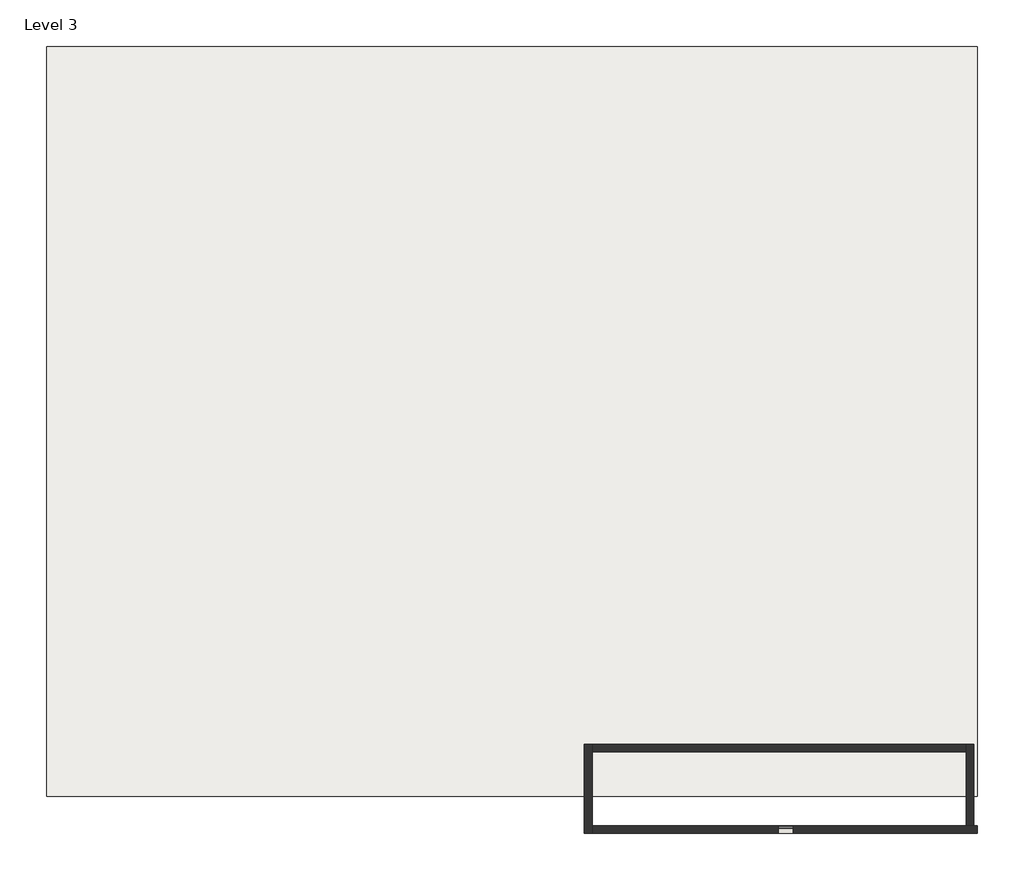
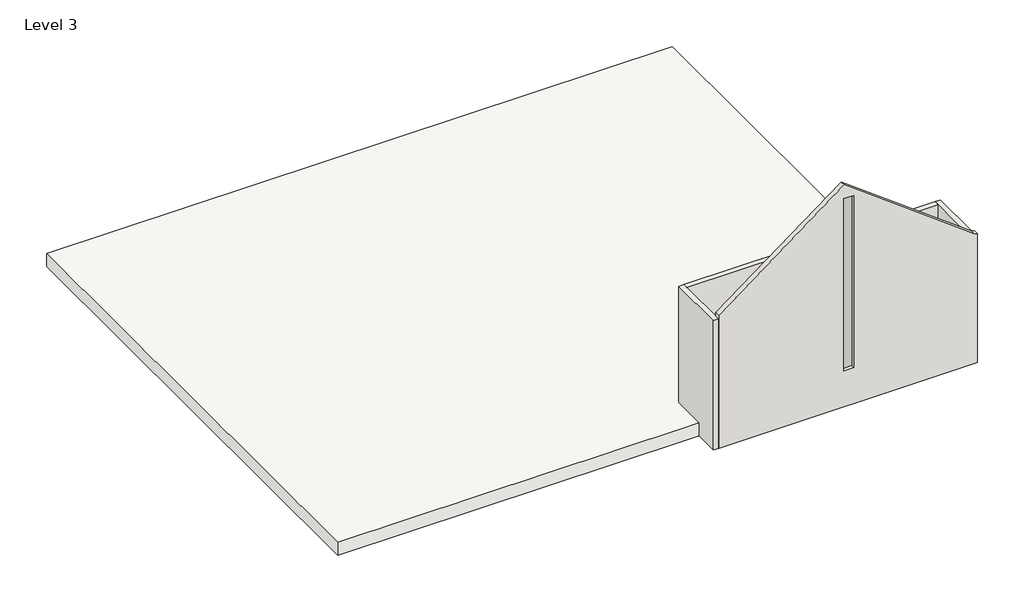
# One storey: 4 walls, 1 plate, 1 roof.
"""IFC4 building model written with IfcOpenShell, lengths in millimetres."""

from ifc_helpers import new_model, si_unit, frame, origin, place, context, project, spatial, polyline, outline, extrude, faceted_brep, transform, mapped, element, save
from components import system_panel_glazed_5b01c733

model = new_model("IFC4")

# Units and contexts
model_context = context("Model", 3, world=origin())
ifc_project = project(units=[si_unit("LENGTHUNIT", "METRE", prefix="MILLI")], contexts=[model_context])

# Site, building, storey
site = spatial("IfcSite", under=ifc_project)
building = spatial("IfcBuilding", under=site)
storey = spatial("IfcBuildingStorey", under=building, Name="Level 3", Elevation=6096.0)

# Plate
placement = place(None, origin())
system_panel_glazed_shape = system_panel_glazed_5b01c733(model_context)
element("IfcPlate", 1, ObjectType="System Panel : Glazed", at=placement, inside=storey, context=model_context, shape_type="MappedRepresentation", body=[
    mapped(system_panel_glazed_shape, transform((-7448.4831929, -10781.7592534, 6942.1825879), x_axis=(1.0, 0.0, 0.0), y_axis=(0.0, 1.0, 0.0), z_axis=(0.0, 0.0, 1.0))),
])

# Roof
element("IfcRoof", 2, ObjectType="Generic - 12\"", at=placement, inside=storey, context=model_context, shape_type="SweptSolid", body=[
    extrude(outline(polyline([(-18522.8831929, 953.0407466), (-4578.2831929, 953.0407466), (-4578.2831929, -10286.4592534), (-18522.8831929, -10286.4592534), (-18522.8831929, 953.0407466)])), frame((0.0, 0.0, 6096.0), z_axis=(0.0, 0.0, 1.0), x_axis=(1.0, 0.0, 0.0)), (0.0, 0.0, 1.0), 304.8),
])

# Walls
element("IfcWall", 3, ObjectType="4.5\"", at=placement, inside=storey, context=model_context, shape_type="Brep", body=[
    faceted_brep([(-10350.4331929, -10838.9092534, 6096.0), (-10350.4331929, -10724.6092534, 6096.0), (-10350.4331929, -9619.7092534, 6096.0), (-10350.4331929, -9505.4092534, 6096.0), (-10350.4331929, -9505.4092534, 9144.0), (-10350.4331929, -9619.7092534, 9144.0), (-10350.4331929, -10838.9092534, 9144.0), (-10464.7331929, -10838.9092534, 6096.0), (-10464.7331929, -10838.9092534, 9144.0), (-10464.7331929, -9505.4092534, 9144.0), (-10464.7331929, -9505.4092534, 6096.0)], [[[0, 1, 2, 3, 4, 5, 6]], [[7, 8, 9, 10]], [[3, 2, 1, 0, 7, 10]], [[6, 5, 4, 9, 8]], [[0, 6, 8, 7]], [[4, 3, 10, 9]]]),
])
element("IfcWall", 4, ObjectType="4.5\"", at=placement, inside=storey, context=model_context, shape_type="Brep", body=[
    faceted_brep([(-4578.2831929, -10724.6092534, 6096.0), (-4635.4331929, -10724.6092534, 6096.0), (-4749.7331929, -10724.6092534, 6096.0), (-10350.4331929, -10724.6092534, 6096.0), (-10350.4331929, -10724.6092534, 9229.725), (-7550.0831929, -10724.6092534, 11329.9875), (-4635.4331929, -10724.6092534, 9144.0), (-4578.2831929, -10724.6092534, 9144.0), (-7562.7831929, -10724.6092534, 11004.5295922), (-7562.7831929, -10724.6092534, 6942.1825879), (-7334.1831929, -10724.6092534, 6942.1825879), (-7334.1831929, -10724.6092534, 11004.5295922), (-10350.4331929, -10838.9092534, 6096.0), (-4578.2831929, -10838.9092534, 6096.0), (-4578.2831929, -10838.9092534, 9144.0), (-4635.4331929, -10838.9092534, 9144.0), (-7550.0831929, -10838.9092534, 11329.9875), (-10350.4331929, -10838.9092534, 9229.725), (-10350.4331929, -10838.9092534, 9144.0), (-7562.7831929, -10838.9092534, 6942.1825879), (-7562.7831929, -10838.9092534, 11004.5295922), (-7334.1831929, -10838.9092534, 11004.5295922), (-7334.1831929, -10838.9092534, 6942.1825879)], [[[0, 1, 2, 3, 4, 5, 6, 7], [8, 9, 10, 11]], [[12, 13, 14, 15, 16, 17, 18], [19, 20, 21, 22]], [[3, 2, 1, 0, 13, 12]], [[0, 7, 14, 13]], [[4, 3, 12, 18, 17]], [[14, 7, 6, 15]], [[6, 5, 16, 15]], [[4, 17, 16, 5]], [[19, 9, 8, 20]], [[20, 8, 11, 21]], [[21, 11, 10, 22]], [[9, 19, 22, 10]]]),
])
element("IfcWall", 5, ObjectType="4.5\"", at=placement, inside=storey, context=model_context, shape_type="Brep", body=[
    faceted_brep([(-4635.4331929, -10724.6092534, 6096.0), (-4635.4331929, -9505.4092534, 6096.0), (-4635.4331929, -9505.4092534, 9144.0), (-4635.4331929, -10724.6092534, 9144.0), (-4749.7331929, -10724.6092534, 6096.0), (-4749.7331929, -10724.6092534, 9144.0), (-4749.7331929, -9619.7092534, 9144.0), (-4749.7331929, -9505.4092534, 9144.0), (-4749.7331929, -9505.4092534, 6096.0), (-4749.7331929, -9619.7092534, 6096.0)], [[[0, 1, 2, 3]], [[4, 5, 6, 7, 8, 9]], [[1, 0, 4, 9, 8]], [[3, 2, 7, 6, 5]], [[0, 3, 5, 4]], [[2, 1, 8, 7]]]),
])
element("IfcWall", 6, ObjectType="4.5\"", at=placement, inside=storey, context=model_context, shape_type="SweptSolid", body=[
    extrude(outline(polyline([(-10350.4331929, -9505.4092534), (-4749.7331929, -9505.4092534), (-4749.7331929, -9619.7092534), (-10350.4331929, -9619.7092534), (-10350.4331929, -9505.4092534)])), frame((0.0, 0.0, 6096.0), z_axis=(0.0, 0.0, 1.0), x_axis=(1.0, 0.0, 0.0)), (0.0, 0.0, 1.0), 3048.0),
])

save(model, "model.ifc")

# Revit data of these elements
# Type "System Panel : Glazed"
#   Construction Type Id = "GSP4R"
#   Analytic Construction = "1/8 in Pilkington single glazing"
#   Visual Light Transmittance = 0.9
#   Solar Heat Gain Coefficient = 0.86
#   Heat Transfer Coefficient (U) = 1.18115 BTU/(h·ft²·°F)
#   Define Thermal Properties by = 1
# Type "Generic - 12\""
#   Assembly Code = "B1020"
#   Layers, outside or top first: 1' - 0" no material (function 1)
# Type "4.5\""
#   Assembly Code = "B2010"
#   Layers, outside or top first: 0' - 4 1/2" no material (function 1)
# Element 1 (IfcPlate, "System Panel : Glazed")
#   Phase Created = New Construction
#   Materials on its faces: "Glass"
# Element 2 (IfcRoof, "Generic - 12\"")
#   built-in parameter 1001705 = 21 (stored number, unit not read)
#   built-in parameter 1001710 = 33615
#   Phase Created = New Construction
#   Materials on its faces: "Default Roof"
# Elements 3, 4, 5, 6 (IfcWall, "4.5\"")
#   Top Offset = 0' - 0"
#   Base Offset = 0' - 0"
#   Unconnected Height = 10' - 0"
#   wall height = 10' - 0"
#   Phase Created = New Construction
#   Base Constraint = Level 3
#   Materials on its faces: "Default Wall"
# Materials
#   "Glass": class "Glass", colour RGB 0 128 192, transparency 0.75, Description = "Soda Lime Glass", Cost = 0
#   "Default Roof": colour RGB 88 101 114, transparency 0, Cost = 0
#   "Default Wall": colour RGB 128 128 128, transparency 0, Cost = 0
